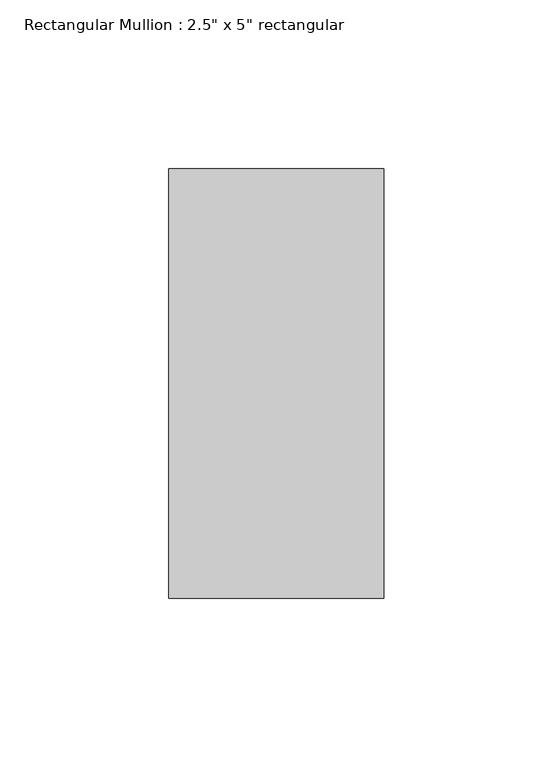
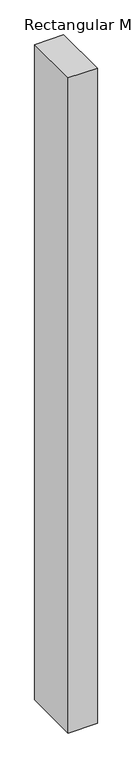
"""IFC4 building model written with IfcOpenShell, lengths in millimetres: member geometry."""

from ifc_helpers import new_model, si_unit, frame, origin, place, context, project, spatial, polyline, outline, extrude, source, transform, mapped, element, save


def member_c224591e(model_context):
    return source(origin(), model_context, "Body", "SweptSolid", [
        extrude(outline(polyline([(31.75, 63.5), (31.75, -63.5), (-31.75, -63.5), (-31.75, 63.5), (31.75, 63.5)])), frame((0.0, 0.0, -1513.786396), z_axis=(0.0, 0.0, 1.0), x_axis=(1.0, 0.0, 0.0)), (0.0, 0.0, 1.0), 1513.786396),
    ])


if __name__ == "__main__":
    model = new_model("IFC4")
    model_context = context("Model", 3, world=origin())
    ifc_project = project(units=[si_unit("LENGTHUNIT", "METRE", prefix="MILLI")], contexts=[model_context])
    site = spatial("IfcSite", under=ifc_project)
    building = spatial("IfcBuilding", under=site)
    placement = place(None, origin())
    member_shape = member_c224591e(model_context)
    element("IfcMember", 1, ObjectType="Rectangular Mullion : 2.5\" x 5\" rectangular", at=placement, inside=building, context=model_context, shape_type="MappedRepresentation", body=[
        mapped(member_shape, transform((0.0, 0.0, 0.0), x_axis=(1.0, 0.0, 0.0), y_axis=(0.0, 1.0, 0.0), z_axis=(0.0, 0.0, 1.0))),
    ])
    save(model, "model.ifc")

# Revit data of these elements
# Type "Rectangular Mullion : 2.5\" x 5\" rectangular"
#   built-in parameter 1007304 = 0.416667 (stored number, unit not read)
#   built-in parameter 1007301 = 0.104167 (stored number, unit not read)
#   built-in parameter 1007300 = 0.104167 (stored number, unit not read)
# Element 1 (IfcMember, "Rectangular Mullion : 2.5\" x 5\" rectangular")
#   Materials on its faces: "Aluminum"
# Materials
#   "Aluminum": class "Metal", colour RGB 247 247 247, transparency 0, Description = "Aluminum 6061", Cost = 0
